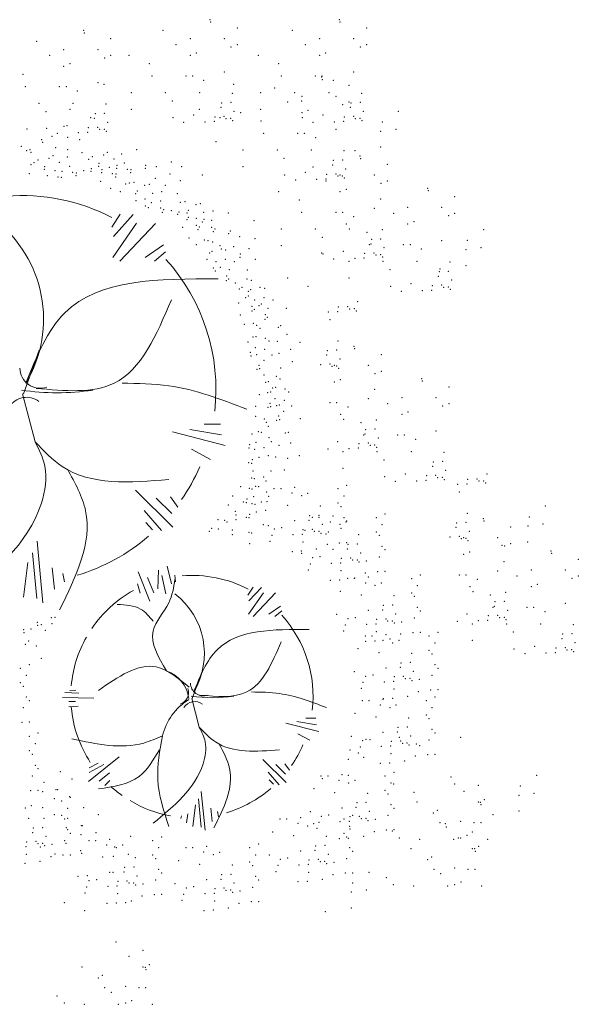
# Model space of a CAD drawing. Units: inches. Extents: x 1239 to 2276906, y 2273 to 321338.
# Tile 23 of 23: x 2272170 to 2276906, y 312990 to 321338. Entities that reach past the tile are written whole.
import ezdxf

# ---------------------------------------------------------------- set-up
doc = ezdxf.new("R2010")
doc.units = ezdxf.units.IN
doc.layers.add('L-PLNT', color=94, linetype='Continuous', lineweight=13)

# ---------------------------------------------------------------- blocks, each defined once
blk = doc.blocks.new('A$C30B31857')
for p, q in [((3.7503, 4.8792), (3.8028, 4.9604)), ((3.7602, 4.8213), (3.8844, 4.9577)), ((3.7571, 4.688), (3.9054, 4.9034)), ((3.8017, 4.6661), (4.0258, 4.9023)), ((3.9592, 4.6879), (4.0761, 4.7684)), ((4.0192, 4.6658), (4.0886, 4.7234)), ((3.1958, 3.8318), (3.2938, 4.1078)), ((3.1896, 3.8318), (3.2693, 3.5312)), ((4.4619, 3.5087), (4.1316, 3.5937)), ((4.4386, 3.5753), (4.2411, 3.6098)), ((4.4331, 3.6423), (4.3299, 3.6433)), ((4.3707, 3.4211), (4.2509, 3.485)), ((4.1343, 2.9958), (3.8994, 3.2279)), ((4.1284, 3.0819), (4.0285, 3.1775)), ((4.1656, 3.1221), (4.1189, 3.1852)), ((4.0628, 2.975), (3.9547, 3.1008)), ((4.0069, 2.9798), (3.9644, 3.0251)), ((3.3185, 2.5196), (3.2812, 2.9071)), ((3.2801, 2.5477), (3.2528, 2.8343)), ((3.196, 2.5571), (3.224, 2.7743)), ((3.39, 2.6068), (3.3766, 2.7403)), ((4.0388, 2.6092), (4.0438, 2.7263)), ((4.1263, 2.6395), (4.0978, 2.7511)), ((3.4532, 2.6516), (3.4426, 2.7052)), ((3.9897, 2.5318), (3.9158, 2.7153)), ((4.0155, 2.5826), (3.975, 2.6798)), ((4.0896, 2.578), (4.065, 2.6912)), ((4.1506, 2.6527), (4.1457, 2.6942)), ((3.928, 2.5823), (3.9112, 2.6389)), ((4.6056, 2.5687), (4.6384, 2.6195)), ((4.6118, 2.5325), (4.6895, 2.6178)), ((4.6098, 2.4492), (4.7026, 2.5839)), ((4.6377, 2.4355), (4.7778, 2.5831)), ((4.7362, 2.4491), (4.8093, 2.4995)), ((4.7737, 2.4353), (4.8171, 2.4714)), ((4.256, 1.9202), (4.3148, 2.0859)), ((3.4418, 1.9254), (3.6381, 1.9223)), ((3.4556, 1.9575), (3.5427, 1.954)), ((3.488, 1.9706), (3.5256, 1.9718)), ((4.2523, 1.9202), (4.3001, 1.7399)), ((3.4801, 1.8674), (3.5393, 1.8722)), ((3.4804, 1.9008), (3.5234, 1.9004)), ((5.0324, 1.7957), (4.9679, 1.7963)), ((5.0504, 1.7122), (4.8439, 1.7653)), ((5.0358, 1.7538), (4.9124, 1.7754)), ((4.9934, 1.6574), (4.9185, 1.6973)), ((3.6033, 1.3996), (3.7969, 1.5536)), ((3.608, 1.4856), (3.6648, 1.5146)), ((3.6093, 1.4548), (3.7012, 1.505)), ((4.8456, 1.3916), (4.6988, 1.5367)), ((4.8419, 1.4454), (4.7795, 1.5052)), ((4.8652, 1.4705), (4.836, 1.51)), ((3.6717, 1.4005), (3.7356, 1.4536)), ((4.8009, 1.3786), (4.7333, 1.4572)), ((3.7064, 1.3744), (3.739, 1.4052)), ((4.766, 1.3816), (4.7394, 1.4099)), ((4.3358, 1.094), (4.3124, 1.3362)), ((4.2592, 1.1174), (4.2766, 1.2532)), ((4.3117, 1.1115), (4.2947, 1.2906)), ((4.1844, 1.1665), (4.1872, 1.1826)), ((4.2206, 1.1393), (4.2277, 1.1957)), ((4.3805, 1.1485), (4.3721, 1.2319)), ((4.4199, 1.1765), (4.4133, 1.21))]:
    blk.add_line(p, q)
for centre, radius, start, end in [((3.1873, 3.861), 1.217, 62.40199, 94.67087), ((2.5377, 4.3028), 0.7844, 329.07822, 52.6009), ((3.1873, 3.861), 1.217, 353.50541, 42.09121), ((3.3005, 3.9951), 0.1272, 180.26687, 289.21544), ((3.4071, 5.3392), 1.4997, 261.42775, 278.57225), ((3.2157, 3.6838), 0.1272, 52.7337, 148.31892), ((3.1873, 3.861), 1.217, 325.31812, 336.41917), ((3.1873, 3.861), 1.217, 286.50052, 310.70203), ((4.2538, 1.9324), 0.7606, 62.40199, 94.67087), ((4.2538, 1.9324), 0.7606, 118.93501, 145.86797), ((3.8611, 2.2029), 0.4706, 329.07822, 52.6009), ((4.2538, 1.9324), 0.7606, 353.50541, 42.09121), ((4.2538, 1.9324), 0.7606, 150.59537, 174.9599), ((4.0258, 1.8951), 0.2096, 6.88406, 70.93506), ((4.153, 1.9587), 0.0795, 289.21544, 17.13172), ((4.3245, 2.0162), 0.0795, 180.26687, 289.21544), ((4.2203, 1.9258), 0.0795, 179.43656, 180.26687), ((4.3827, 2.8247), 0.8998, 261.42775, 278.57225), ((4.2538, 1.9324), 0.7606, 185.11549, 212.96103), ((4.4263, 1.5995), 0.3678, 121.54331, 166.60172), ((4.2715, 1.8216), 0.0795, 52.7337, 148.31892), ((4.2538, 1.9324), 0.7606, 325.31812, 336.41917), ((4.2538, 1.9324), 0.7606, 227.99389, 234.92066), ((4.2538, 1.9324), 0.7606, 286.50052, 310.70203), ((4.2538, 1.9324), 0.7606, 239.25491, 259.86097)]:
    blk.add_arc(centre, radius, start, end)
for points, knots in [([(3.2106, 3.8997), (3.2782, 4.0657), (3.478, 4.5561), (4.0445, 4.5549), (4.4191, 4.5541)], [0, 0, 0, 0, 0.505063, 1.491803, 1.491803, 1.491803, 1.491803]), ([(3.2759, 3.867), (3.4546, 3.8509), (3.8645, 3.8139), (4.0311, 4.2035), (4.1251, 4.4232)], [0, 0, 0, 0, 0.49103, 1.125938, 1.125938, 1.125938, 1.125938]), ([(3.8148, 3.8997), (3.9136, 3.8984), (4.1838, 3.8949), (4.4376, 3.7978), (4.5987, 3.7361)], [0, 0, 0, 0, 0.29442, 0.8060024, 0.8060024, 0.8060024, 0.8060024]), ([(3.2693, 3.5312), (3.2945, 3.4812), (3.355, 3.361), (3.2868, 2.9371), (3.0051, 2.7057), (2.786, 2.5256)], [0, 0, 0, 0, 0.165135, 0.396758, 1.208872, 1.208872, 1.208872, 1.208872]), ([(3.2693, 3.5312), (3.3234, 3.4742), (3.5366, 3.2499), (3.8644, 3.2754), (4.1088, 3.2945)], [0, 0, 0, 0, 0.229976, 0.9045396, 0.9045396, 0.9045396, 0.9045396]), ([(3.4719, 3.3599), (3.5196, 3.2734), (3.6746, 2.9922), (3.5259, 2.6875), (3.4229, 2.4766)], [0, 0, 0, 0, 0.2856103, 0.9283265, 0.9283265, 0.9283265, 0.9283265]), ([(4.0943, 2.0932), (4.0431, 2.1794), (3.9528, 2.3314), (4.1194, 2.5003), (4.1389, 2.6174), (4.1473, 2.6677)], [0, 0, 0, 0, 0.2643394, 0.4663641, 0.6187177, 0.6187177, 0.6187177, 0.6187177]), ([(4.0102, 2.4054), (3.986, 2.4345), (3.9287, 2.5035), (3.8375, 2.508), (3.7847, 2.5106)], [0, 0, 0, 0, 0.1091589, 0.2590609, 0.2590609, 0.2590609, 0.2590609]), ([(4.2649, 1.961), (4.3054, 2.0606), (4.4253, 2.3548), (4.7652, 2.3541), (4.99, 2.3536)], [0, 0, 0, 0, 0.303038, 0.8950819, 0.8950819, 0.8950819, 0.8950819]), ([(4.3041, 1.9414), (4.4113, 1.9317), (4.6572, 1.9095), (4.7572, 2.1433), (4.8136, 2.2751)], [0, 0, 0, 0, 0.2946182, 0.675563, 0.675563, 0.675563, 0.675563]), ([(4.2355, 1.9904), (4.1681, 2.0469), (3.9917, 2.1946), (3.7911, 2.0563), (3.6671, 1.9708)], [0, 0, 0, 0, 0.2421239, 0.6334325, 0.6334325, 0.6334325, 0.6334325]), ([(4.6274, 1.961), (4.6866, 1.9602), (4.8488, 1.9581), (5.0011, 1.8998), (5.0978, 1.8629)], [0, 0, 0, 0, 0.176652, 0.4836014, 0.4836014, 0.4836014, 0.4836014]), ([(4.3001, 1.7399), (4.3152, 1.7099), (4.3515, 1.6377), (4.3106, 1.3834), (4.1416, 1.2446), (4.0101, 1.1365)], [0, 0, 0, 0, 0.0990809, 0.2380551, 0.7253232, 0.7253232, 0.7253232, 0.7253232]), ([(4.3001, 1.7399), (4.3326, 1.7057), (4.4604, 1.5711), (4.6571, 1.5864), (4.8038, 1.5978)], [0, 0, 0, 0, 0.1379856, 0.5427238, 0.5427238, 0.5427238, 0.5427238]), ([(4.0689, 1.6862), (4.0299, 1.669), (3.8517, 1.5906), (3.6546, 1.6333), (3.5005, 1.6666)], [0, 0, 0, 0, 0.1264411, 0.5776247, 0.5776247, 0.5776247, 0.5776247]), ([(4.0689, 1.6862), (4.0518, 1.5941), (4.0159, 1.4014), (4.0764, 1.2145), (4.1081, 1.1169)], [0, 0, 0, 0, 0.2763889, 0.5787232, 0.5787232, 0.5787232, 0.5787232]), ([(4.4216, 1.6371), (4.4503, 1.5852), (4.5433, 1.4165), (4.454, 1.2337), (4.3922, 1.1071)], [0, 0, 0, 0, 0.1713662, 0.5569959, 0.5569959, 0.5569959, 0.5569959]), ([(4.0493, 1.5978), (4.0122, 1.5345), (3.928, 1.3908), (3.7607, 1.3662), (3.6671, 1.3525)], [0, 0, 0, 0, 0.2099222, 0.4765171, 0.4765171, 0.4765171, 0.4765171])]:
    blk.add_open_spline(points, degree=3, knots=knots)
for p in [(4.3671, 6.1817), (5.1793, 6.1817), (4.3711, 6.1664), (4.5382, 6.1295), (5.1833, 6.1664), (5.3504, 6.1295), (3.5734, 6.1141), (3.5774, 6.0988), (3.7445, 6.0619), (4.0717, 6.1142), (4.2428, 6.062), (4.4567, 6.062), (4.8839, 6.1142), (5.055, 6.062), (5.2689, 6.062), (3.278, 6.0466), (4.1532, 6.025), (4.4994, 6.0098), (4.5382, 6.025), (4.9654, 6.025), (5.3116, 6.0098), (5.3504, 6.025), (3.3595, 5.9574), (3.4491, 5.9944), (3.6629, 5.9944), (3.7057, 5.9422), (3.7445, 5.9574), (3.8578, 5.9575), (4.2428, 5.9575), (4.2816, 5.9728), (4.67, 5.9575), (5.055, 5.9575), (5.0937, 5.9728), (3.4491, 5.8899), (3.4878, 5.9052), (3.9861, 5.9053), (4.7983, 5.9053), (3.1924, 5.8377), (4.002, 5.8283), (4.2159, 5.8283), (4.2586, 5.8283), (4.4567, 5.8531), (4.8142, 5.8283), (5.0281, 5.8283), (5.0685, 5.8211), (5.0708, 5.8283), (5.2689, 5.8531), (3.2083, 5.7607), (3.4221, 5.7607), (3.4649, 5.7607), (3.6629, 5.7855), (3.7026, 5.7761), (4.3283, 5.8008), (4.5148, 5.7761), (4.7731, 5.7537), (5.0726, 5.8059), (5.1405, 5.8008), (5.2396, 5.7689), (3.5346, 5.7332), (3.8737, 5.7238), (4.0876, 5.7238), (4.3014, 5.7238), (4.507, 5.7196), (4.6859, 5.7238), (4.8997, 5.7238), (4.9442, 5.7014), (5.1136, 5.7238), (5.1581, 5.7014), (5.3192, 5.7196), (3.2938, 5.6562), (3.5077, 5.6562), (3.7133, 5.652), (4.1303, 5.6716), (4.4356, 5.6305), (4.44, 5.6593), (4.4982, 5.662), (4.8547, 5.6645), (4.9425, 5.6716), (5.2009, 5.6492), (5.2396, 5.6645), (5.2478, 5.6305), (5.2522, 5.6593), (5.3104, 5.662), (3.3366, 5.604), (3.4887, 5.6194), (3.617, 5.5672), (3.6463, 5.5917), (3.7045, 5.5944), (3.8737, 5.6194), (4.1351, 5.5664), (4.2638, 5.5831), (4.3009, 5.6194), (4.3977, 5.5715), (4.4292, 5.5672), (4.4559, 5.5742), (4.5185, 5.6058), (4.5593, 5.597), (4.6859, 5.6194), (4.9442, 5.597), (4.9473, 5.5664), (4.983, 5.6122), (5.076, 5.5831), (5.2099, 5.5715), (5.2681, 5.5742), (5.3307, 5.6058), (5.5495, 5.607), (3.4498, 5.5125), (3.4701, 5.5155), (3.604, 5.5039), (3.6419, 5.5629), (3.6622, 5.5066), (3.7248, 5.5382), (4.2026, 5.5364), (4.3351, 5.54), (4.3933, 5.5427), (4.4683, 5.5605), (4.4974, 5.5619), (4.5097, 5.5482), (4.6876, 5.5447), (5.0148, 5.5364), (5.1473, 5.54), (5.2055, 5.5427), (5.2804, 5.5605), (5.3095, 5.5619), (5.3219, 5.5482), (5.4484, 5.5393), (3.2183, 5.4955), (3.3414, 5.4988), (3.3754, 5.4495), (3.4088, 5.4688), (3.4726, 5.4423), (3.5414, 5.4724), (3.5996, 5.4751), (3.6745, 5.4929), (3.7036, 5.4943), (3.716, 5.4806), (4.7034, 5.4677), (4.9173, 5.4677), (4.9601, 5.4677), (5.0298, 5.4403), (5.1581, 5.4925), (5.4396, 5.4817), (5.5341, 5.4943), (3.1825, 5.3868), (3.3111, 5.4286), (3.3168, 5.4111), (3.3983, 5.3793), (3.5483, 5.4281), (4.404, 5.4155), (5.4388, 5.3816), (3.2153, 5.3587), (3.2368, 5.3657), (3.2368, 5.3657), (3.2425, 5.3481), (3.3807, 5.3283), (3.4704, 5.3189), (3.474, 5.3651), (3.5639, 5.3462), (3.6293, 5.3208), (3.6985, 5.3321), (3.7228, 5.3481), (3.8125, 5.3386), (3.906, 5.3659), (4.5751, 5.3633), (4.789, 5.3633), (5.0029, 5.3633), (5.2085, 5.359), (5.2765, 5.3597), (5.3085, 5.3254), (3.2439, 5.2709), (3.2628, 5.2851), (3.2872, 5.3011), (3.3282, 5.2596), (3.3564, 5.3123), (3.4217, 5.2869), (3.487, 5.2615), (3.6049, 5.3048), (3.6683, 5.261), (3.6703, 5.2794), (3.7638, 5.3066), (3.7823, 5.2676), (3.8291, 5.2812), (3.9636, 5.2671), (4.0309, 5.26), (4.1244, 5.2873), (4.1902, 5.2588), (4.5751, 5.2588), (4.8318, 5.3111), (5.0131, 5.2579), (5.137, 5.2699), (5.1414, 5.2987), (5.1997, 5.3014), (5.3125, 5.3101), (5.4796, 5.2732), (3.2327, 5.214), (3.3262, 5.2413), (3.3448, 5.2022), (3.3935, 5.2342), (3.4121, 5.1951), (3.4345, 5.1928), (3.4383, 5.2295), (3.5056, 5.2224), (3.5261, 5.2017), (3.528, 5.2201), (3.528, 5.2201), (3.5748, 5.2337), (3.6196, 5.229), (3.6216, 5.2474), (3.6869, 5.2219), (3.6888, 5.2403), (3.7356, 5.2539), (3.7541, 5.2149), (3.7746, 5.1942), (3.7766, 5.2125), (3.7804, 5.2492), (3.8477, 5.2421), (3.8682, 5.2214), (3.8701, 5.2398), (3.8701, 5.2398), (3.9617, 5.2487), (4.1167, 5.2139), (4.3185, 5.2066), (4.8366, 5.2059), (4.9652, 5.2226), (5.0991, 5.2109), (5.1573, 5.2137), (5.1697, 5.2), (5.1842, 5.2057), (5.1988, 5.2013), (5.2199, 5.2452), (5.3981, 5.2057), (3.6811, 5.1669), (3.838, 5.1504), (3.8611, 5.1556), (3.8899, 5.1603), (3.9577, 5.1424), (3.9864, 5.1471), (4.0232, 5.1866), (4.0866, 5.1428), (4.1801, 5.1701), (4.904, 5.1758), (5.0365, 5.1794), (5.0946, 5.1687), (5.0947, 5.1821), (5.2111, 5.1876), (5.4408, 5.1534), (5.4796, 5.1687), (3.7445, 5.1231), (3.8047, 5.1029), (3.9012, 5.0898), (3.9105, 5.1058), (4.007, 5.0926), (4.0645, 5.1021), (4.1611, 5.0889), (4.7992, 5.1012), (5.1842, 5.1012), (5.223, 5.1165), (5.7331, 5.1226), (5.7371, 5.1073), (5.9042, 5.0703), (3.9023, 5.0465), (3.9598, 5.056), (3.9609, 5.0127), (3.9989, 5.0334), (4.0564, 5.0428), (4.1817, 5.0344), (4.2104, 5.0391), (4.2782, 5.0213), (4.3069, 5.026), (4.9275, 5.049), (5.4376, 5.0551), (3.9804, 5.0015), (4.0574, 4.9996), (4.0677, 4.9724), (4.0769, 4.9883), (4.0769, 4.9883), (4.1252, 4.9818), (4.1643, 4.9592), (4.1735, 4.9752), (4.2218, 4.9687), (4.231, 4.9846), (4.3275, 4.9715), (4.385, 4.9809), (4.4816, 4.9678), (4.9434, 4.972), (5.1573, 4.972), (5.2, 4.972), (5.3981, 4.9967), (5.5192, 4.9659), (5.6087, 5.0028), (5.8226, 5.0028), (5.8654, 4.9506), (5.9042, 4.9659), (4.2228, 4.9254), (4.2321, 4.9414), (4.2803, 4.9348), (4.2814, 4.8916), (4.3194, 4.9123), (4.3286, 4.9283), (4.3769, 4.9217), (4.644, 4.9198), (5.2238, 4.8984), (5.2697, 4.9445), (5.6087, 4.8984), (5.6475, 4.9136), (4.1951, 4.8775), (4.2917, 4.8644), (4.3009, 4.8803), (4.3779, 4.8785), (4.3882, 4.8512), (4.3975, 4.8672), (4.3975, 4.8672), (4.4848, 4.8381), (4.494, 4.8541), (4.8151, 4.8675), (5.029, 4.8675), (5.2428, 4.8675), (5.3521, 4.8462), (5.4484, 4.8633), (6.0848, 4.8633), (4.2353, 4.8117), (4.282, 4.7688), (4.3318, 4.7986), (4.355, 4.7939), (4.3832, 4.7865), (4.4301, 4.7631), (4.5526, 4.8203), (4.6491, 4.8072), (4.8151, 4.7631), (5.0717, 4.8153), (5.368, 4.7692), (5.377, 4.7741), (5.3814, 4.8029), (5.4396, 4.8057), (5.5818, 4.7692), (5.6246, 4.7692), (5.8226, 4.7939), (5.9837, 4.7957), (4.3649, 4.7175), (4.3798, 4.7283), (4.4379, 4.7427), (4.4661, 4.7353), (4.5157, 4.7564), (4.5584, 4.7108), (4.6122, 4.7432), (5.0685, 4.7169), (5.0765, 4.7101), (5.2052, 4.7268), (5.3391, 4.7152), (5.3973, 4.7179), (5.4097, 4.7042), (5.4388, 4.7056), (5.4599, 4.7495), (5.6943, 4.7417), (5.9749, 4.7381), (6.0694, 4.7506), (4.3483, 4.6776), (4.4047, 4.6628), (4.4627, 4.6771), (4.5191, 4.6623), (4.5558, 4.6906), (4.6523, 4.6775), (5.144, 4.6801), (5.2396, 4.6647), (5.2765, 4.6836), (5.3347, 4.6864), (5.4511, 4.6919), (5.4535, 4.6647), (5.6674, 4.6647), (5.873, 4.6605), (5.9741, 4.638), (4.388, 4.6229), (4.4013, 4.6046), (4.4312, 4.6263), (4.4875, 4.6115), (4.6019, 4.6111), (5.4963, 4.6125), (5.806, 4.6001), (5.8118, 4.616), (5.8642, 4.6029), (4.4692, 4.5425), (4.4709, 4.5716), (4.4842, 4.5534), (4.4842, 4.5534), (4.5256, 4.5277), (4.5986, 4.5529), (4.6267, 4.5455), (4.8547, 4.5603), (5.2396, 4.5603), (5.6298, 4.524), (5.8016, 4.5713), (5.8219, 4.5151), (5.8845, 4.5466), (4.5521, 4.4913), (4.567, 4.5021), (4.6085, 4.4765), (4.6234, 4.4873), (4.6814, 4.5016), (4.7096, 4.4942), (4.983, 4.508), (5.5011, 4.5073), (5.5685, 4.4772), (5.701, 4.4808), (5.7593, 4.4836), (5.7637, 4.5124), (5.8342, 4.5014), (5.8633, 4.5028), (5.8757, 4.489), (4.547, 4.404), (4.5918, 4.4366), (4.6068, 4.4474), (4.6482, 4.4218), (4.6896, 4.3961), (4.7062, 4.4361), (4.7626, 4.4213), (5.2938, 4.4114), (4.5569, 4.3276), (4.6299, 4.3528), (4.6316, 4.3818), (4.6448, 4.3636), (4.6747, 4.3853), (4.7145, 4.3306), (4.7311, 4.3705), (4.8455, 4.37), (5.1104, 4.3456), (5.1686, 4.3484), (5.173, 4.3772), (5.2312, 4.3799), (5.2435, 4.3662), (5.2726, 4.3675), (5.285, 4.3538), (4.5822, 4.2693), (4.6398, 4.2763), (4.7128, 4.3015), (4.7277, 4.3123), (4.7277, 4.3123), (5.1212, 4.2982), (4.6591, 4.2626), (4.6818, 4.2444), (4.7956, 4.2502), (4.8106, 4.2611), (4.8503, 4.2064), (4.6056, 4.1591), (4.6371, 4.1888), (4.6551, 4.1927), (4.714, 4.1821), (4.7367, 4.1639), (4.7906, 4.163), (4.9332, 4.1551), (5.1715, 4.1647), (4.6197, 4.0929), (4.6511, 4.1227), (4.71, 4.1121), (4.8005, 4.0866), (4.8735, 4.1117), (5.1045, 4.1044), (5.1627, 4.1071), (5.2716, 4.131), (5.2756, 4.1158), (4.6244, 4.0709), (4.6605, 4.0786), (4.706, 4.0421), (4.7554, 4.0757), (4.8833, 4.0353), (5.1001, 4.0756), (5.1204, 4.0193), (5.183, 4.0509), (5.4427, 4.0788), (4.6612, 3.9865), (4.6746, 4.0124), (4.6792, 3.9904), (4.6792, 3.9904), (4.8103, 3.9952), (5.0622, 4.0166), (5.1328, 4.0056), (5.1473, 4.0113), (5.1619, 4.007), (5.1742, 3.9933), (5.3611, 4.0113), (5.4039, 3.9591), (5.4427, 3.9743), (4.7067, 3.9501), (4.716, 3.906), (4.7341, 3.9098), (4.7836, 3.9434), (4.8063, 3.9252), (5.1473, 3.9069), (5.186, 3.9221), (5.6961, 3.9282), (5.7001, 3.913), (4.7301, 3.8399), (4.7482, 3.8437), (4.7615, 3.8696), (4.7796, 3.8734), (4.8384, 3.8629), (4.8612, 3.8447), (5.4007, 3.8607), (5.8672, 3.876), (4.6759, 3.8283), (4.7442, 3.7737), (4.7756, 3.8034), (4.8344, 3.7929), (5.1204, 3.7776), (5.1631, 3.7776), (5.3611, 3.8024), (5.4823, 3.7715), (5.5718, 3.8085), (5.7857, 3.8085), (5.8672, 3.7715), (4.6539, 3.7545), (4.7308, 3.7478), (4.7489, 3.7517), (4.785, 3.7593), (4.803, 3.7632), (4.8304, 3.7229), (4.8799, 3.7565), (5.2328, 3.7502), (5.6106, 3.7193), (5.8285, 3.7563), (4.6533, 3.691), (4.7088, 3.674), (4.7208, 3.6536), (4.7857, 3.6673), (4.799, 3.6932), (4.8037, 3.6711), (4.8037, 3.6711), (4.9348, 3.6759), (5.1869, 3.704), (5.2059, 3.6732), (5.3152, 3.6518), (5.4115, 3.6689), (5.5718, 3.704), (4.6707, 3.5951), (4.6887, 3.5913), (4.7342, 3.6277), (4.8405, 3.5868), (4.8586, 3.5906), (5.3445, 3.6086), (5.4027, 3.6113), (5.7857, 3.5996), (4.6299, 3.5808), (4.6566, 3.529), (4.7382, 3.5578), (4.7515, 3.5319), (4.8726, 3.5245), (5.1683, 3.5325), (5.331, 3.5748), (5.3401, 3.5798), (5.423, 3.5551), (5.5449, 3.5748), (5.5877, 3.5748), (5.6574, 3.5474), (4.6111, 3.4926), (4.6158, 3.5146), (4.6472, 3.4849), (4.7061, 3.4954), (4.8004, 3.5091), (5.1071, 3.4857), (5.2027, 3.4704), (5.2396, 3.4893), (5.2978, 3.492), (5.3022, 3.5208), (5.3604, 3.5236), (5.3727, 3.5099), (5.4018, 3.5112), (5.4142, 3.4975), (5.4166, 3.4704), (5.6305, 3.4704), (5.8361, 3.4661), (4.6104, 3.4005), (4.6332, 3.4187), (4.674, 3.4331), (4.7328, 3.4437), (4.7784, 3.4353), (4.8553, 3.4286), (4.9275, 3.4439), (5.4594, 3.4181), (5.769, 3.4058), (5.8273, 3.4085), (4.6285, 3.3967), (4.6285, 3.3967), (4.6372, 3.3488), (4.7502, 3.3478), (4.8332, 3.3548), (5.2027, 3.3659), (5.7646, 3.377), (5.8475, 3.3523), (4.6278, 3.3047), (4.6458, 3.3008), (4.7047, 3.3114), (4.718, 3.2855), (5.4642, 3.3129), (5.5316, 3.2829), (5.5928, 3.3297), (5.6641, 3.2865), (5.7223, 3.2892), (5.7267, 3.318), (5.7849, 3.3208), (5.7973, 3.307), (5.8264, 3.3084), (5.8387, 3.2947), (5.9852, 3.2955), (6.0434, 3.2982), (6.0557, 3.2845), (6.0848, 3.2859), (6.106, 3.3298), (4.5596, 3.25), (4.6137, 3.2385), (4.6318, 3.2347), (4.6545, 3.2529), (4.6726, 3.2491), (4.722, 3.2155), (4.7696, 3.2368), (4.8124, 3.2368), (4.8997, 3.2451), (5.1707, 3.2366), (5.2261, 3.2591), (5.9226, 3.2639), (5.9334, 3.2165), (5.9808, 3.2667), (6.0972, 3.2722), (4.5094, 3.1915), (4.5769, 3.1541), (4.5997, 3.1724), (4.6404, 3.1867), (4.6899, 3.1532), (4.7246, 3.1559), (4.7354, 3.1896), (4.8821, 3.2093), (4.9424, 3.1929), (4.9812, 3.2082), (5.2076, 3.1915), (4.483, 3.1338), (4.5268, 3.0957), (4.595, 3.1503), (4.6311, 3.1426), (4.6491, 3.1388), (4.6578, 3.0909), (4.7167, 3.1014), (4.8552, 3.1323), (5.0608, 3.1281), (5.1707, 3.1464), (5.1892, 3.1239), (6.4724, 3.1281), (4.4168, 3.0426), (4.4599, 3.0391), (4.5295, 3.0722), (4.5312, 3.0431), (4.5943, 3.0583), (4.6123, 3.0544), (4.6123, 3.0544), (4.617, 3.0765), (4.8997, 3.0362), (4.9894, 3.039), (4.9938, 3.0678), (5.0096, 3.0565), (5.052, 3.0705), (5.0524, 3.0565), (5.1221, 3.0291), (5.1396, 3.0649), (5.2076, 3.0562), (5.2261, 3.0337), (5.4107, 3.0563), (5.4661, 3.0788), (5.9837, 3.083), (6.0838, 3.0494), (6.0878, 3.0341), (6.3714, 3.0605), (4.3638, 2.9696), (4.377, 2.9879), (4.4201, 2.9844), (4.4748, 3.0283), (4.5064, 2.9775), (4.7017, 3.0115), (4.734, 3.0055), (4.7714, 2.984), (4.8176, 2.9916), (4.9515, 2.98), (4.9645, 2.9757), (5.0097, 2.9827), (5.022, 2.969), (5.0511, 2.9704), (5.0723, 3.0143), (5.1824, 3.0126), (5.1892, 2.9886), (5.2212, 3.0279), (5.4476, 3.0112), (5.9123, 2.9939), (5.9167, 3.0227), (5.9749, 3.0254), (5.9952, 2.9692), (6.2549, 2.9971), (6.3626, 3.0029), (6.4571, 3.0154), (4.508, 2.9484), (4.6116, 2.9624), (4.6297, 2.9586), (4.7444, 2.907), (4.7563, 2.9449), (4.8889, 2.9485), (4.9471, 2.9512), (5.0635, 2.9567), (5.0952, 2.9521), (5.1094, 2.9645), (5.3008, 2.9478), (5.4107, 2.9661), (5.4292, 2.9436), (5.8744, 2.9349), (5.9326, 2.9377), (5.945, 2.9239), (5.9595, 2.9296), (5.9741, 2.9253), (5.9864, 2.9116), (6.1733, 2.9296), (4.6156, 2.8924), (4.9412, 2.8452), (4.95, 2.9027), (5.0357, 2.8577), (5.1032, 2.8877), (5.1396, 2.8559), (5.1798, 2.8972), (5.2261, 2.8984), (5.2293, 2.8587), (5.2337, 2.8875), (5.2919, 2.8902), (5.4476, 2.8759), (5.4661, 2.8534), (6.1994, 2.8809), (6.2161, 2.8774), (6.2549, 2.8927), (6.3617, 2.9028), (6.5083, 2.8465), (4.883, 2.8424), (4.9416, 2.8312), (5.0113, 2.8037), (5.0575, 2.8114), (5.1914, 2.7997), (5.2496, 2.8025), (5.262, 2.7887), (5.2911, 2.7901), (5.3122, 2.834), (5.3494, 2.7842), (5.4292, 2.8083), (5.9595, 2.8252), (5.9982, 2.8404), (6.5123, 2.8313), (6.6794, 2.7943), (4.9844, 2.7267), (4.9963, 2.7646), (5.1288, 2.7682), (5.187, 2.7709), (5.19, 2.7225), (5.3034, 2.7764), (6.1733, 2.7207), (6.2129, 2.7791), (6.384, 2.7268), (6.5979, 2.7268), (5.123, 2.6621), (5.1812, 2.6649), (5.2311, 2.6734), (5.2739, 2.6734), (5.2757, 2.6774), (5.3431, 2.7074), (5.3611, 2.6818), (5.4198, 2.7169), (5.4661, 2.7181), (5.6322, 2.6732), (5.6876, 2.6957), (5.9325, 2.696), (5.9753, 2.696), (6.045, 2.6685), (6.2945, 2.6899), (6.6407, 2.6746), (6.6794, 2.6899), (5.3436, 2.646), (5.4039, 2.6295), (5.4427, 2.6448), (5.6691, 2.6281), (5.999, 2.6224), (6.384, 2.6224), (6.4228, 2.6376), (5.186, 2.5926), (5.3167, 2.569), (5.5223, 2.5647), (5.6322, 2.583), (5.6507, 2.5605), (6.0181, 2.5915), (6.1274, 2.5701), (6.2237, 2.5873), (5.3611, 2.4728), (5.4508, 2.4756), (5.4552, 2.5044), (5.5135, 2.5071), (5.6691, 2.4929), (6.1432, 2.4932), (6.1523, 2.4981), (6.1567, 2.5269), (6.2149, 2.5297), (6.2352, 2.4734), (6.3571, 2.4932), (6.3999, 2.4932), (6.5979, 2.5179), (3.371, 2.4265), (3.3934, 2.4288), (5.1631, 2.4481), (5.2328, 2.4206), (5.279, 2.4283), (5.4129, 2.4166), (5.4711, 2.4194), (5.5337, 2.4509), (5.6507, 2.4252), (5.6876, 2.4703), (5.9805, 2.4508), (6.1144, 2.4392), (6.1726, 2.4419), (6.1849, 2.4282), (6.214, 2.4296), (6.2264, 2.4158), (6.4696, 2.4657), (3.1974, 2.3525), (3.2423, 2.3573), (3.2832, 2.3987), (3.2852, 2.3803), (3.2852, 2.3803), (3.3076, 2.3827), (3.3748, 2.3897), (5.2178, 2.3815), (5.3503, 2.3851), (5.4085, 2.3878), (5.4835, 2.4056), (5.5126, 2.407), (5.5249, 2.3933), (5.5709, 2.4011), (5.9192, 2.404), (6.0149, 2.3887), (6.0518, 2.4076), (6.11, 2.4104), (6.2288, 2.3887), (6.4426, 2.3887), (6.6482, 2.3844), (3.1994, 2.3342), (3.3339, 2.3483), (5.2059, 2.3436), (5.3419, 2.3129), (5.3846, 2.3129), (5.4115, 2.3394), (5.4719, 2.3212), (5.4972, 2.2943), (5.5646, 2.3243), (5.6413, 2.3338), (5.6876, 2.3351), (5.743, 2.3126), (5.7983, 2.3352), (6.2715, 2.3365), (6.5768, 2.2953), (6.5812, 2.3241), (6.6394, 2.3268), (3.2071, 2.2608), (3.2276, 2.2815), (3.2763, 2.2495), (5.2968, 2.232), (5.3445, 2.279), (5.4027, 2.2818), (5.4543, 2.2854), (5.5147, 2.269), (5.5534, 2.2842), (5.7799, 2.2676), (6.0149, 2.2842), (6.2764, 2.2313), (6.405, 2.248), (6.5389, 2.2363), (6.5971, 2.2391), (6.6386, 2.2267), (6.6597, 2.2706), (3.3085, 2.1726), (5.4274, 2.2084), (5.633, 2.2042), (5.743, 2.2225), (5.7614, 2.1999), (6.3438, 2.2012), (6.4763, 2.2048), (6.5345, 2.2075), (6.6095, 2.2254), (6.6509, 2.213), (3.1772, 2.1098), (3.2325, 2.1324), (5.4719, 2.1123), (5.5616, 2.115), (5.566, 2.1438), (5.6242, 2.1466), (5.7799, 2.1323), (5.7983, 2.1098), (3.2141, 2.0647), (5.2739, 2.0875), (5.3436, 2.0601), (5.3898, 2.0677), (5.5237, 2.0561), (5.5819, 2.0588), (5.5942, 2.0451), (5.6233, 2.0465), (5.6445, 2.0903), (5.6816, 2.0406), (5.7614, 2.0647), (3.1772, 2.0197), (3.1956, 1.9971), (5.3167, 1.9831), (5.3286, 2.0209), (5.4611, 2.0245), (5.5193, 2.0273), (5.5223, 1.9788), (5.6357, 2.0327), (3.2141, 1.9295), (5.4552, 1.9185), (5.5135, 1.9212), (5.608, 1.9338), (5.6754, 1.9638), (5.752, 1.9732), (5.7799, 1.9296), (5.7983, 1.9745), (3.1956, 1.8619), (3.2325, 1.9069), (5.3234, 1.9072), (5.3662, 1.9072), (5.4359, 1.8798), (5.4534, 1.9156), (5.4962, 1.8633), (5.535, 1.8786), (5.7245, 1.907), (5.7614, 1.8619), (5.2783, 1.8264), (5.409, 1.8028), (5.6146, 1.7985), (5.7245, 1.8168), (5.743, 1.7943), (3.1862, 1.7704), (3.2325, 1.7717), (5.5475, 1.7382), (5.6057, 1.7409), (3.2326, 1.6817), (3.2879, 1.7042), (5.2554, 1.6819), (5.4534, 1.7067), (5.5431, 1.7094), (5.5561, 1.6758), (5.626, 1.6847), (5.7614, 1.7267), (5.7799, 1.7041), (5.9411, 1.6758), (3.2695, 1.6366), (5.3101, 1.6153), (5.3251, 1.6544), (5.3465, 1.6634), (5.3713, 1.6621), (5.4426, 1.6189), (5.5008, 1.6216), (5.5052, 1.6504), (5.5634, 1.6532), (5.5758, 1.6395), (5.6049, 1.6408), (5.6172, 1.6271), (5.6632, 1.635), (5.6844, 1.6236), (5.743, 1.659), (3.2326, 1.5915), (3.251, 1.569), (5.2454, 1.5957), (5.2982, 1.5774), (5.3311, 1.5507), (5.5038, 1.5732), (5.6569, 1.5582), (5.7336, 1.5676), (5.7799, 1.5689), (3.2695, 1.5013), (5.2366, 1.5381), (5.4368, 1.5129), (5.495, 1.5156), (5.5895, 1.5281), (3.251, 1.4337), (3.2879, 1.4788), (3.4267, 1.4606), (5.065, 1.434), (5.1078, 1.434), (5.195, 1.4423), (5.2357, 1.438), (5.4661, 1.4338), (5.5214, 1.4563), (5.8807, 1.427), (6.4171, 1.438), (3.3257, 1.3929), (3.5006, 1.4155), (5.0734, 1.4161), (5.1774, 1.4065), (5.2378, 1.3901), (5.2766, 1.4054), (5.503, 1.3887), (5.5192, 1.3828), (5.9042, 1.3828), (6.0518, 1.3747), (6.316, 1.3704), (3.2416, 1.3422), (3.2879, 1.3435), (3.3169, 1.3353), (3.3995, 1.3478), (3.4114, 1.3479), (3.4852, 1.3028), (3.491, 1.2986), (5.0199, 1.3531), (5.1505, 1.3296), (5.3561, 1.3253), (5.4661, 1.3436), (5.4845, 1.3211), (5.6475, 1.3306), (5.9622, 1.3378), (6.3072, 1.3128), (6.4017, 1.3253), (3.2461, 1.2476), (3.3907, 1.2902), (3.4356, 1.276), (5.2891, 1.265), (5.3473, 1.2677), (5.503, 1.2534), (5.6668, 1.2703), (6.0518, 1.2703), (6.0653, 1.2691), (6.0693, 1.2539), (6.0905, 1.2855), (3.2073, 1.2324), (3.316, 1.2352), (3.3898, 1.1901), (3.4356, 1.1859), (3.4725, 1.231), (3.5744, 1.2352), (3.6667, 1.1901), (4.997, 1.2087), (5.0667, 1.1812), (5.1129, 1.1889), (5.195, 1.2334), (5.2468, 1.1772), (5.263, 1.1859), (5.2847, 1.2362), (5.305, 1.1799), (5.3676, 1.2115), (5.4845, 1.1858), (5.5214, 1.2309), (5.7699, 1.2016), (5.7951, 1.2181), (6.1441, 1.1907), (6.3063, 1.2127), (3.2276, 1.1682), (3.3257, 1.1676), (3.4541, 1.1633), (3.4733, 1.1676), (3.559, 1.1225), (3.5656, 1.1225), (4.8066, 1.1636), (4.8493, 1.1636), (4.919, 1.1361), (4.9366, 1.1719), (4.9794, 1.1197), (5.0181, 1.135), (5.0517, 1.1421), (5.1842, 1.1457), (5.2077, 1.1634), (5.2424, 1.1484), (5.2446, 1.1183), (5.3174, 1.1662), (5.3465, 1.1676), (5.3588, 1.1539), (5.4047, 1.1617), (5.811, 1.1411), (5.8437, 1.134), (5.941, 1.1494), (6.0248, 1.1411), (6.0676, 1.1411), (3.2542, 1.0784), (3.2586, 1.1072), (3.3169, 1.11), (3.3371, 1.0537), (3.4645, 1.11), (3.4725, 1.0957), (3.491, 1.0732), (3.5568, 1.0649), (3.6513, 1.0774), (3.8698, 1.0549), (4.7615, 1.0827), (4.8921, 1.0591), (5.0398, 1.1042), (5.0977, 1.0549), (5.2077, 1.0732), (5.2454, 1.1), (5.3311, 1.0549), (5.3985, 1.0849), (5.4751, 1.0944), (5.5115, 1.0888), (5.5214, 1.0956), (5.8514, 1.1124), (5.9798, 1.0602), (6.0148, 1.0818), (3.2119, 0.9907), (3.2163, 1.0195), (3.2745, 1.0222), (3.2869, 1.0085), (3.316, 1.0099), (3.3283, 0.9961), (3.3743, 1.004), (3.4541, 1.0281), (3.4637, 1.0099), (3.6067, 1.0284), (3.6495, 1.0284), (3.7192, 1.0009), (3.7368, 1.0367), (3.8183, 0.9997), (4.0078, 1.0282), (4.0632, 1.0507), (4.3459, 0.9916), (4.6723, 1.0056), (5.0307, 0.9946), (5.0889, 0.9973), (5.1784, 1.0396), (5.2261, 1.0506), (5.2366, 1.0424), (5.556, 1.0449), (5.6826, 1.0366), (5.8965, 1.0366), (5.9253, 1.0448), (5.941, 1.0449), (6.0536, 0.9926), (6.1104, 1.0366), (3.2149, 0.9422), (3.3014, 0.9879), (3.3937, 0.9429), (3.4447, 0.9366), (3.491, 0.9379), (3.556, 0.9648), (3.5617, 0.9475), (3.7599, 0.9297), (3.7687, 0.9873), (3.7795, 0.9845), (3.8544, 0.9422), (4.0078, 0.938), (4.0447, 0.9831), (4.2159, 0.9833), (4.2586, 0.9833), (4.3283, 0.9559), (4.3887, 0.9394), (4.4274, 0.9547), (4.617, 0.9831), (4.6539, 0.938), (4.7386, 0.9382), (4.9366, 0.963), (5.0263, 0.9658), (5.1092, 0.9411), (5.2446, 0.983), (5.263, 0.9605), (5.6299, 0.9773), (6.0148, 0.9773), (6.0284, 0.9762), (6.0324, 0.9609), (3.2061, 0.8846), (3.3006, 0.8972), (3.368, 0.9272), (3.6923, 0.9239), (3.8979, 0.9197), (4.0263, 0.9154), (4.1708, 0.9024), (4.3014, 0.8789), (4.507, 0.8746), (4.617, 0.8929), (4.6354, 0.8704), (4.7933, 0.8717), (4.8083, 0.9108), (4.8545, 0.9184), (4.9258, 0.8753), (4.984, 0.878), (4.9884, 0.9068), (5.0466, 0.9095), (5.0589, 0.8958), (5.088, 0.8972), (5.1004, 0.8835), (5.1463, 0.8913), (5.2261, 0.9154), (5.733, 0.9087), (5.7582, 0.9251), (3.5967, 0.8076), (3.7368, 0.8278), (3.759, 0.8296), (3.8265, 0.8305), (3.8309, 0.8593), (3.8891, 0.8621), (3.9094, 0.8059), (4.0447, 0.8478), (4.0632, 0.8253), (4.44, 0.8143), (4.4982, 0.817), (4.7814, 0.8338), (4.987, 0.8295), (5.1401, 0.8145), (5.2167, 0.8239), (5.263, 0.8252), (5.3649, 0.8296), (5.774, 0.8481), (5.8145, 0.8195), (5.9041, 0.8564), (5.9879, 0.8481), (6.0307, 0.8481), (3.5388, 0.803), (3.6084, 0.7756), (3.6547, 0.7832), (3.7842, 0.7428), (3.7886, 0.7716), (3.8468, 0.7743), (3.8591, 0.7606), (3.8882, 0.762), (3.9006, 0.7483), (3.9465, 0.7561), (4.0263, 0.7802), (4.1479, 0.758), (4.3459, 0.7827), (4.4356, 0.7855), (4.5185, 0.7608), (4.6539, 0.8027), (4.6723, 0.7802), (4.9199, 0.7692), (4.9781, 0.7719), (5.0727, 0.7845), (5.2638, 0.7619), (5.4746, 0.7959), (5.5191, 0.752), (5.6457, 0.7436), (5.8596, 0.7436), (5.9041, 0.752), (5.9428, 0.7672), (6.0735, 0.7436), (3.5815, 0.6986), (3.5934, 0.7365), (3.726, 0.74), (3.7871, 0.6943), (4.0169, 0.6887), (4.0632, 0.69), (4.2026, 0.6914), (4.2176, 0.7305), (4.2638, 0.7382), (4.3351, 0.695), (4.3933, 0.6977), (4.3977, 0.7265), (4.4559, 0.7293), (4.4683, 0.7155), (4.4974, 0.7169), (4.5097, 0.7032), (4.5556, 0.711), (4.6354, 0.7351), (5.255, 0.7043), (5.3495, 0.7169), (3.4518, 0.6392), (3.7201, 0.634), (3.7783, 0.6367), (3.8368, 0.6392), (3.8728, 0.6493), (3.9403, 0.6793), (4.1907, 0.6535), (4.3963, 0.6493), (4.5494, 0.6342), (4.626, 0.6437), (4.6723, 0.6449), (3.5801, 0.587), (4.3293, 0.5889), (4.3875, 0.5917), (4.482, 0.6042), (5.0919, 0.5823), (5.2542, 0.6042), (3.7764, 0.3904), (3.9475, 0.3381), (3.8579, 0.3012), (3.9862, 0.2489), (3.5625, 0.2337), (3.9475, 0.2337), (3.961, 0.2325), (3.965, 0.2172), (3.6656, 0.165), (3.6908, 0.1815), (3.7067, 0.1045), (3.7471, 0.0758), (3.8367, 0.1128), (3.9205, 0.1045), (3.9633, 0.1045), (3.4072, 0.0522), (3.4517, 0.0083), (3.5783, 0), (3.7922, 0), (3.8367, 0.0083), (3.8755, 0.0236), (4.0061, 0)]:
    blk.add_point(p)
blk = doc.blocks.new('p2')
at = {"xscale": 1000, "yscale": 1000, "zscale": 1000}
blk.add_blockref('A$C30B31857', (-714.2, -1628.3), dxfattribs=at)

msp = doc.modelspace()

# ---------------------------------------------------------------- block references
at = {"layer": 'L-PLNT', "xscale": 1.35042108782907, "yscale": 1.35042108782907, "zscale": 1.35042108782907}
msp.add_blockref('p2', (2268850.67, 315188.45), dxfattribs=at)

doc.saveas('drawing.dxf')
